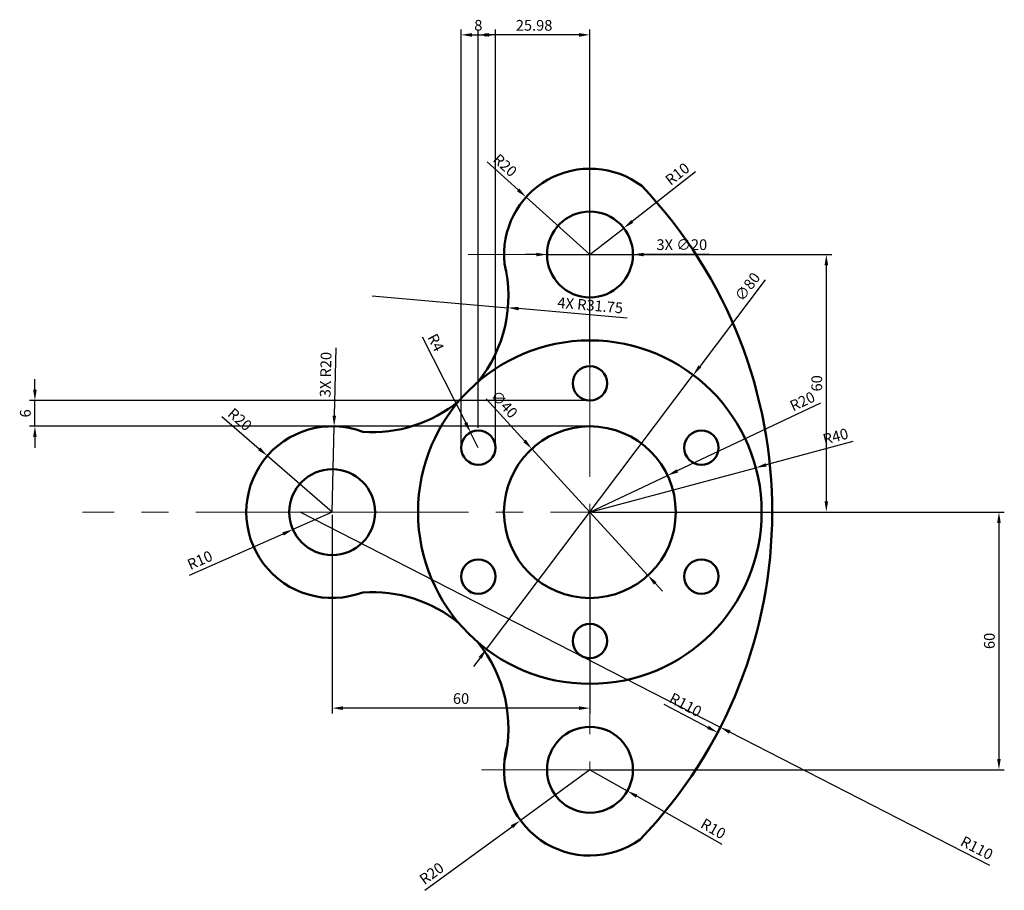
# Model space of a CAD drawing. Units: millimetres. Extents: x 4193 to 4422, y 3154 to 3357.
import ezdxf

# ---------------------------------------------------------------- set-up
doc = ezdxf.new("R2010")
doc.units = ezdxf.units.MM
doc.linetypes.add('CENTER', pattern=[50.8, 31.75, -6.35, 6.35, -6.35])
for name, color, linetype, lineweight in [('M-CNTR', 4, 'CENTER', 18), ('M-DIMS', 2, 'Continuous', 25), ('M-OUTL', 7, 'Continuous', 50)]:
    doc.layers.add(name, color=color, linetype=linetype, lineweight=lineweight)
doc.styles.get("Standard").update_dxf_attribs({"font": 'arial.ttf'})
doc.dimstyles.new('ISO-25', dxfattribs={"dimtxt": 2.5, "dimasz": 2.5, "dimexe": 1.25, "dimexo": 0.625, "dimtad": 1, "dimtxsty": 'Standard', "dimcen": 2.5, "dimadec": 0, "dimazin": 0, "dimtfac": 1, "dimtmove": 0, "dimatfit": 3, "dimfxl": 1, "dimarcsym": 0})

# ---------------------------------------------------------------- blocks, each defined once
blk = doc.blocks.new('*U1')
blk.add_circle((0, 0), 4)
blk = doc.blocks.new('*U2')
at = {"layer": 'M-OUTL', "color": 0, "linetype": 'ByBlock', "lineweight": -2, "transparency": 16777216}
for p, rotation in [((4325.57, 3272.51), 180), ((4299.59, 3257.51), 240), ((4351.55, 3257.51), 119.9999999999999), ((4299.59, 3227.51), 300), ((4351.55, 3227.51), 59.99999999999997)]:
    blk.add_blockref('*U1', p, dxfattribs=dict(at, rotation=rotation))
blk.add_blockref('*U1', (4325.57, 3212.51), dxfattribs=at)
blk = doc.blocks.new('*D3')
at = {"layer": 'Defpoints', "color": 0, "transparency": 16777216}
for p in [(4325.57, 3242.51), (4325.59, 3182.51), (4420.83, 3182.51)]:
    blk.add_point(p, dxfattribs=at)
at = {"layer": 'M-DIMS', "color": 0, "lineweight": -2, "transparency": 16777216}
for p, q in [((4326.2, 3242.51), (4422.08, 3242.51)), ((4420.83, 3240.01), (4420.83, 3185.01)), ((4326.22, 3182.51), (4422.08, 3182.51))]:
    blk.add_line(p, q, dxfattribs=at)
at = {"layer": 'M-DIMS', "color": 0, "transparency": 16777216}
for points in [[(4420.41, 3240.01), (4421.24, 3240.01), (4420.83, 3242.51)], [(4420.41, 3185.01), (4421.24, 3185.01), (4420.83, 3182.51)]]:
    blk.add_solid(points, dxfattribs=at)
at = {"layer": 'M-DIMS', "color": 0, "transparency": 16777216, "insert": (4418.92, 3212.51), "char_height": 2.5, "attachment_point": 5, "rotation": 90}
blk.add_mtext('60', dxfattribs=at)
blk = doc.blocks.new('*D4')
at = {"layer": 'Defpoints', "color": 0, "transparency": 16777216}
for p in [(4265.57, 3242.51), (4325.57, 3242.51), (4265.57, 3196.86)]:
    blk.add_point(p, dxfattribs=at)
at = {"layer": 'M-DIMS', "color": 0, "lineweight": -2, "transparency": 16777216}
for p, q in [((4265.57, 3241.88), (4265.57, 3195.61)), ((4325.57, 3241.88), (4325.57, 3195.61)), ((4323.07, 3196.86), (4268.07, 3196.86))]:
    blk.add_line(p, q, dxfattribs=at)
at = {"layer": 'M-DIMS', "color": 0, "transparency": 16777216}
for points in [[(4268.07, 3197.27), (4268.07, 3196.44), (4265.57, 3196.86)], [(4323.07, 3197.27), (4323.07, 3196.44), (4325.57, 3196.86)]]:
    blk.add_solid(points, dxfattribs=at)
at = {"layer": 'M-DIMS', "color": 0, "transparency": 16777216, "insert": (4295.57, 3198.76), "char_height": 2.5, "attachment_point": 5}
blk.add_mtext('60', dxfattribs=at)
blk = doc.blocks.new('*D5')
at = {"layer": 'Defpoints', "color": 0, "transparency": 16777216}
for p in [(4333.46, 3308.67), (4325.59, 3302.51)]:
    blk.add_point(p, dxfattribs=at)
at = {"layer": 'M-DIMS', "color": 0, "lineweight": -2, "transparency": 16777216}
for p, q in [((4350.15, 3321.75), (4335.43, 3310.22)), ((4325.59, 3302.51), (4333.46, 3308.67))]:
    blk.add_line(p, q, dxfattribs=at)
at = {"layer": 'M-DIMS', "color": 0, "transparency": 16777216}
blk.add_solid([(4335.18, 3310.54), (4335.69, 3309.89), (4333.46, 3308.67)], dxfattribs=at)
at = {"layer": 'M-DIMS', "color": 0, "transparency": 16777216, "insert": (4346.14, 3321.02), "char_height": 2.5, "attachment_point": 5, "rotation": 38.0842}
blk.add_mtext('R10', dxfattribs=at)
blk = doc.blocks.new('*D6')
at = {"layer": 'Defpoints', "color": 0, "transparency": 16777216}
for p in [(4310.73, 3315.89), (4325.59, 3302.51)]:
    blk.add_point(p, dxfattribs=at)
at = {"layer": 'M-DIMS', "color": 0, "lineweight": -2, "transparency": 16777216}
for p, q in [((4301.65, 3324.06), (4308.87, 3317.56)), ((4325.59, 3302.51), (4310.73, 3315.89))]:
    blk.add_line(p, q, dxfattribs=at)
at = {"layer": 'M-DIMS', "color": 0, "transparency": 16777216}
blk.add_solid([(4309.15, 3317.87), (4308.59, 3317.25), (4310.73, 3315.89)], dxfattribs=at)
at = {"layer": 'M-DIMS', "color": 0, "transparency": 16777216, "insert": (4305.6, 3323.06), "char_height": 2.5, "attachment_point": 5, "rotation": 318.016}
blk.add_mtext('R20', dxfattribs=at)
blk = doc.blocks.new('*D7')
at = {"layer": 'Defpoints', "color": 0, "transparency": 16777216}
for p in [(4364.21, 3252.86), (4325.57, 3242.51)]:
    blk.add_point(p, dxfattribs=at)
at = {"layer": 'M-DIMS', "color": 0, "lineweight": -2, "transparency": 16777216}
for p, q in [((4386.84, 3258.93), (4366.62, 3253.51)), ((4325.57, 3242.51), (4364.21, 3252.86))]:
    blk.add_line(p, q, dxfattribs=at)
at = {"layer": 'M-DIMS', "color": 0, "transparency": 16777216}
blk.add_solid([(4366.51, 3253.91), (4366.73, 3253.11), (4364.21, 3252.86)], dxfattribs=at)
at = {"layer": 'M-DIMS', "color": 0, "transparency": 16777216, "insert": (4382.86, 3259.83), "char_height": 2.5, "attachment_point": 5, "rotation": 15.0027}
blk.add_mtext('R40', dxfattribs=at)
blk = doc.blocks.new('*D8')
at = {"layer": 'Defpoints', "color": 0, "transparency": 16777216}
for p in [(4343.66, 3251.04), (4325.57, 3242.51)]:
    blk.add_point(p, dxfattribs=at)
at = {"layer": 'M-DIMS', "color": 0, "lineweight": -2, "transparency": 16777216}
for p, q in [((4379.26, 3267.85), (4345.92, 3252.11)), ((4325.57, 3242.51), (4343.66, 3251.04))]:
    blk.add_line(p, q, dxfattribs=at)
at = {"layer": 'M-DIMS', "color": 0, "transparency": 16777216}
blk.add_solid([(4345.74, 3252.49), (4346.1, 3251.73), (4343.66, 3251.04)], dxfattribs=at)
at = {"layer": 'M-DIMS', "color": 0, "transparency": 16777216, "insert": (4375.19, 3268.03), "char_height": 2.5, "attachment_point": 5, "rotation": 25.2677}
blk.add_mtext('R20', dxfattribs=at)
blk = doc.blocks.new('*D9')
at = {"layer": 'Defpoints', "color": 0, "transparency": 16777216}
for p in [(4297.79, 3261.08), (4299.59, 3257.51)]:
    blk.add_point(p, dxfattribs=at)
at = {"layer": 'M-DIMS', "color": 0, "lineweight": -2, "transparency": 16777216}
for p, q in [((4286.54, 3283.36), (4296.66, 3263.31)), ((4299.59, 3257.51), (4297.79, 3261.08))]:
    blk.add_line(p, q, dxfattribs=at)
at = {"layer": 'M-DIMS', "color": 0, "transparency": 16777216}
blk.add_solid([(4297.03, 3263.5), (4296.29, 3263.12), (4297.79, 3261.08)], dxfattribs=at)
at = {"layer": 'M-DIMS', "color": 0, "transparency": 16777216, "insert": (4289.4, 3281.85), "char_height": 2.5, "attachment_point": 5, "rotation": 296.7817}
blk.add_mtext('R4', dxfattribs=at)
blk = doc.blocks.new('*D10')
at = {"layer": 'Defpoints', "color": 0, "transparency": 16777216}
for p in [(4265.57, 3242.51), (4256.42, 3238.46)]:
    blk.add_point(p, dxfattribs=at)
at = {"layer": 'M-DIMS', "color": 0, "lineweight": -2, "transparency": 16777216}
for p, q in [((4265.57, 3242.51), (4256.42, 3238.46)), ((4232.36, 3227.82), (4254.14, 3237.45))]:
    blk.add_line(p, q, dxfattribs=at)
at = {"layer": 'M-DIMS', "color": 0, "transparency": 16777216}
blk.add_solid([(4253.97, 3237.83), (4254.31, 3237.07), (4256.42, 3238.46)], dxfattribs=at)
at = {"layer": 'M-DIMS', "color": 0, "transparency": 16777216, "insert": (4234.89, 3231.02), "char_height": 2.5, "attachment_point": 5, "rotation": 23.8595}
blk.add_mtext('R10', dxfattribs=at)
blk = doc.blocks.new('*D11')
at = {"layer": 'Defpoints', "color": 0, "transparency": 16777216}
for p in [(4250.46, 3255.61), (4265.57, 3242.51)]:
    blk.add_point(p, dxfattribs=at)
at = {"layer": 'M-DIMS', "color": 0, "lineweight": -2, "transparency": 16777216}
for p, q in [((4239.88, 3264.78), (4248.57, 3257.25)), ((4265.57, 3242.51), (4250.46, 3255.61))]:
    blk.add_line(p, q, dxfattribs=at)
at = {"layer": 'M-DIMS', "color": 0, "transparency": 16777216}
blk.add_solid([(4248.84, 3257.56), (4248.3, 3256.93), (4250.46, 3255.61)], dxfattribs=at)
at = {"layer": 'M-DIMS', "color": 0, "transparency": 16777216, "insert": (4243.86, 3263.85), "char_height": 2.5, "attachment_point": 5, "rotation": 319.0732}
blk.add_mtext('R20', dxfattribs=at)
blk = doc.blocks.new('*D12')
at = {"layer": 'Defpoints', "color": 0, "transparency": 16777216}
for p in [(4258.02, 3242.57), (4355.29, 3191.2)]:
    blk.add_point(p, dxfattribs=at)
at = {"layer": 'M-DIMS', "color": 0, "lineweight": -2, "transparency": 16777216}
blk.add_line((4342.77, 3197.81), (4353.08, 3192.37), dxfattribs=at)
at = {"layer": 'M-DIMS', "color": 0, "transparency": 16777216}
blk.add_solid([(4353.27, 3192.74), (4352.88, 3192), (4355.29, 3191.2)], dxfattribs=at)
at = {"layer": 'M-DIMS', "color": 0, "transparency": 16777216, "insert": (4347.7, 3197.35), "char_height": 2.5, "attachment_point": 5, "rotation": 332.1578}
blk.add_mtext('R110', dxfattribs=at)
blk = doc.blocks.new('*D13')
at = {"layer": 'Defpoints', "color": 0, "transparency": 16777216}
for p in [(4325.59, 3182.51), (4334.29, 3177.57)]:
    blk.add_point(p, dxfattribs=at)
at = {"layer": 'M-DIMS', "color": 0, "lineweight": -2, "transparency": 16777216}
for p, q in [((4325.59, 3182.51), (4334.29, 3177.57)), ((4356.35, 3165.06), (4336.47, 3176.34))]:
    blk.add_line(p, q, dxfattribs=at)
at = {"layer": 'M-DIMS', "color": 0, "transparency": 16777216}
blk.add_solid([(4336.67, 3176.7), (4336.26, 3175.98), (4334.29, 3177.57)], dxfattribs=at)
at = {"layer": 'M-DIMS', "color": 0, "transparency": 16777216, "insert": (4354.15, 3168.5), "char_height": 2.5, "attachment_point": 5, "rotation": 330.4382}
blk.add_mtext('R10', dxfattribs=at)
blk = doc.blocks.new('*D14')
at = {"layer": 'Defpoints', "color": 0, "transparency": 16777216}
for p in [(4325.57, 3182.51), (4309.42, 3170.71)]:
    blk.add_point(p, dxfattribs=at)
at = {"layer": 'M-DIMS', "color": 0, "lineweight": -2, "transparency": 16777216}
for p, q in [((4325.57, 3182.51), (4309.42, 3170.71)), ((4287.1, 3154.42), (4307.4, 3169.24))]:
    blk.add_line(p, q, dxfattribs=at)
at = {"layer": 'M-DIMS', "color": 0, "transparency": 16777216}
blk.add_solid([(4307.15, 3169.58), (4307.64, 3168.9), (4309.42, 3170.71)], dxfattribs=at)
at = {"layer": 'M-DIMS', "color": 0, "transparency": 16777216, "insert": (4288.9, 3158.09), "char_height": 2.5, "attachment_point": 5, "rotation": 36.1328}
blk.add_mtext('R20', dxfattribs=at)
blk = doc.blocks.new('MOUNTING-HOLE-D20')
blk.add_circle((10, 10), 10)
blk = doc.blocks.new('*D16')
at = {"layer": 'Defpoints', "color": 0, "transparency": 16777216}
for p in [(4325.59, 3302.51), (4325.57, 3242.51), (4380.63, 3242.51)]:
    blk.add_point(p, dxfattribs=at)
at = {"layer": 'M-DIMS', "color": 0, "lineweight": -2, "transparency": 16777216}
for p, q in [((4326.22, 3302.51), (4381.88, 3302.51)), ((4380.63, 3300.01), (4380.63, 3245.01)), ((4326.2, 3242.51), (4381.88, 3242.51))]:
    blk.add_line(p, q, dxfattribs=at)
at = {"layer": 'M-DIMS', "color": 0, "transparency": 16777216}
for points in [[(4380.22, 3300.01), (4381.05, 3300.01), (4380.63, 3302.51)], [(4380.22, 3245.01), (4381.05, 3245.01), (4380.63, 3242.51)]]:
    blk.add_solid(points, dxfattribs=at)
at = {"layer": 'M-DIMS', "color": 0, "transparency": 16777216, "insert": (4378.73, 3272.51), "char_height": 2.5, "attachment_point": 5, "rotation": 90}
blk.add_mtext('60', dxfattribs=at)
blk = doc.blocks.new('*D17')
at = {"layer": 'Defpoints', "color": 0, "transparency": 16777216}
for p in [(4196.34, 3268.51), (4325.57, 3268.51), (4325.57, 3262.51)]:
    blk.add_point(p, dxfattribs=at)
at = {"layer": 'M-DIMS', "color": 0, "lineweight": -2, "transparency": 16777216}
for p, q in [((4196.34, 3271.01), (4196.34, 3273.51)), ((4324.95, 3268.51), (4195.09, 3268.51)), ((4196.34, 3262.51), (4196.34, 3268.51)), ((4324.95, 3262.51), (4195.09, 3262.51)), ((4196.34, 3260.01), (4196.34, 3257.51))]:
    blk.add_line(p, q, dxfattribs=at)
at = {"layer": 'M-DIMS', "color": 0, "transparency": 16777216}
for points in [[(4195.92, 3271.01), (4196.75, 3271.01), (4196.34, 3268.51)], [(4195.92, 3260.01), (4196.75, 3260.01), (4196.34, 3262.51)]]:
    blk.add_solid(points, dxfattribs=at)
at = {"layer": 'M-DIMS', "color": 0, "transparency": 16777216, "insert": (4194.43, 3265.51), "char_height": 2.5, "attachment_point": 5, "rotation": 90}
blk.add_mtext('6', dxfattribs=at)
blk = doc.blocks.new('*D18')
at = {"layer": 'Defpoints', "color": 0, "transparency": 16777216}
for p in [(4299.59, 3353.67), (4325.57, 3276.51), (4299.59, 3261.51)]:
    blk.add_point(p, dxfattribs=at)
at = {"layer": 'M-DIMS', "color": 0, "lineweight": -2, "transparency": 16777216}
for p, q in [((4299.59, 3262.13), (4299.59, 3354.92)), ((4325.57, 3277.13), (4325.57, 3354.92)), ((4323.07, 3353.67), (4302.09, 3353.67))]:
    blk.add_line(p, q, dxfattribs=at)
at = {"layer": 'M-DIMS', "color": 0, "transparency": 16777216}
for points in [[(4302.09, 3354.08), (4302.09, 3353.25), (4299.59, 3353.67)], [(4323.07, 3354.08), (4323.07, 3353.25), (4325.57, 3353.67)]]:
    blk.add_solid(points, dxfattribs=at)
at = {"layer": 'M-DIMS', "color": 0, "transparency": 16777216, "insert": (4312.58, 3355.57), "char_height": 2.5, "attachment_point": 5}
blk.add_mtext('25.98', dxfattribs=at)
blk = doc.blocks.new('*D19')
at = {"layer": 'Defpoints', "color": 0, "transparency": 16777216}
for p in [(4303.59, 3353.67), (4295.59, 3257.51), (4303.59, 3257.51)]:
    blk.add_point(p, dxfattribs=at)
at = {"layer": 'M-DIMS', "color": 0, "lineweight": -2, "transparency": 16777216}
for p, q in [((4295.59, 3258.13), (4295.59, 3354.92)), ((4303.59, 3258.13), (4303.59, 3354.92)), ((4298.09, 3353.67), (4301.09, 3353.67))]:
    blk.add_line(p, q, dxfattribs=at)
at = {"layer": 'M-DIMS', "color": 0, "transparency": 16777216}
for points in [[(4298.09, 3354.08), (4298.09, 3353.25), (4295.59, 3353.67)], [(4301.09, 3354.08), (4301.09, 3353.25), (4303.59, 3353.67)]]:
    blk.add_solid(points, dxfattribs=at)
at = {"layer": 'M-DIMS', "color": 0, "transparency": 16777216, "insert": (4299.59, 3355.57), "char_height": 2.5, "attachment_point": 5}
blk.add_mtext('8', dxfattribs=at)
blk = doc.blocks.new('*D20')
at = {"layer": 'Defpoints', "color": 0, "transparency": 16777216}
for p in [(4266, 3262.5), (4265.57, 3242.51)]:
    blk.add_point(p, dxfattribs=at)
at = {"layer": 'M-DIMS', "color": 0, "lineweight": -2, "transparency": 16777216}
for p, q in [((4266.39, 3280.79), (4266.05, 3265)), ((4265.57, 3242.51), (4266, 3262.5))]:
    blk.add_line(p, q, dxfattribs=at)
at = {"layer": 'M-DIMS', "color": 0, "transparency": 16777216}
blk.add_solid([(4265.64, 3265.01), (4266.47, 3264.99), (4266, 3262.5)], dxfattribs=at)
at = {"layer": 'M-DIMS', "color": 0, "transparency": 16777216, "insert": (4264.36, 3274.54), "char_height": 2.5, "attachment_point": 5, "rotation": 88.7678}
blk.add_mtext('3X R20', dxfattribs=at)
blk = doc.blocks.new('*D21')
at = {"layer": 'Defpoints', "color": 0, "transparency": 16777216}
for p in [(4274.85, 3292.87), (4306.48, 3290.12)]:
    blk.add_point(p, dxfattribs=at)
at = {"layer": 'M-DIMS', "color": 0, "lineweight": -2, "transparency": 16777216}
for p, q in [((4274.85, 3292.87), (4306.48, 3290.12)), ((4334.22, 3287.71), (4308.97, 3289.91))]:
    blk.add_line(p, q, dxfattribs=at)
at = {"layer": 'M-DIMS', "color": 0, "transparency": 16777216}
blk.add_solid([(4309.01, 3290.32), (4308.94, 3289.49), (4306.48, 3290.12)], dxfattribs=at)
at = {"layer": 'M-DIMS', "color": 0, "transparency": 16777216, "insert": (4325.63, 3290.37), "char_height": 2.5, "attachment_point": 5, "rotation": 355.0338}
blk.add_mtext('4X R31.75', dxfattribs=at)
blk = doc.blocks.new('*D22')
at = {"layer": 'Defpoints', "color": 0, "transparency": 16777216}
for p in [(4258.02, 3242.57), (4355.92, 3192.42)]:
    blk.add_point(p, dxfattribs=at)
at = {"layer": 'M-DIMS', "color": 0, "lineweight": -2, "transparency": 16777216}
for p, q in [((4258.02, 3242.57), (4355.92, 3192.42)), ((4418.73, 3160.23), (4358.14, 3191.28))]:
    blk.add_line(p, q, dxfattribs=at)
at = {"layer": 'M-DIMS', "color": 0, "transparency": 16777216}
blk.add_solid([(4358.33, 3191.65), (4357.95, 3190.91), (4355.92, 3192.42)], dxfattribs=at)
at = {"layer": 'M-DIMS', "color": 0, "transparency": 16777216, "insert": (4415.53, 3164.01), "char_height": 2.5, "attachment_point": 5, "rotation": 332.8725}
blk.add_mtext('R110', dxfattribs=at)
blk = doc.blocks.new('*D23')
at = {"layer": 'Defpoints', "color": 0, "transparency": 16777216}
for p in [(4315.59, 3302.51), (4335.59, 3302.51)]:
    blk.add_point(p, dxfattribs=at)
at = {"layer": 'M-DIMS', "color": 0, "lineweight": -2, "transparency": 16777216}
for p, q in [((4313.09, 3302.51), (4310.59, 3302.51)), ((4315.59, 3302.51), (4335.59, 3302.51)), ((4353.37, 3302.51), (4338.09, 3302.51))]:
    blk.add_line(p, q, dxfattribs=at)
at = {"layer": 'M-DIMS', "color": 0, "transparency": 16777216}
for points in [[(4313.09, 3302.92), (4313.09, 3302.09), (4315.59, 3302.51)], [(4338.09, 3302.92), (4338.09, 3302.09), (4335.59, 3302.51)]]:
    blk.add_solid(points, dxfattribs=at)
at = {"layer": 'M-DIMS', "color": 0, "transparency": 16777216, "insert": (4346.98, 3304.48), "char_height": 2.5, "attachment_point": 5, "rotation": 0.0026}
blk.add_mtext('3X ∅20', dxfattribs=at)
blk = doc.blocks.new('*D24')
at = {"layer": 'Defpoints', "color": 0, "transparency": 16777216}
for p in [(4312.05, 3257.24), (4339.09, 3227.77)]:
    blk.add_point(p, dxfattribs=at)
at = {"layer": 'M-DIMS', "color": 0, "lineweight": -2, "transparency": 16777216}
for p, q in [((4301.39, 3268.87), (4310.36, 3259.09)), ((4339.09, 3227.77), (4312.05, 3257.24)), ((4340.78, 3225.93), (4342.47, 3224.08))]:
    blk.add_line(p, q, dxfattribs=at)
at = {"layer": 'M-DIMS', "color": 0, "transparency": 16777216}
for points in [[(4310.67, 3259.37), (4310.05, 3258.81), (4312.05, 3257.24)], [(4341.09, 3226.21), (4340.47, 3225.64), (4339.09, 3227.77)]]:
    blk.add_solid(points, dxfattribs=at)
at = {"layer": 'M-DIMS', "color": 0, "transparency": 16777216, "insert": (4305.39, 3267.42), "char_height": 2.5, "attachment_point": 5, "rotation": 312.5304}
blk.add_mtext('∅40', dxfattribs=at)
blk = doc.blocks.new('*D25')
at = {"layer": 'Defpoints', "color": 0, "transparency": 16777216}
for p in [(4349.65, 3274.45), (4301.49, 3210.57)]:
    blk.add_point(p, dxfattribs=at)
at = {"layer": 'M-DIMS', "color": 0, "lineweight": -2, "transparency": 16777216}
for p, q in [((4366.37, 3296.62), (4351.15, 3276.44)), ((4301.49, 3210.57), (4349.65, 3274.45)), ((4299.99, 3208.57), (4298.48, 3206.57))]:
    blk.add_line(p, q, dxfattribs=at)
at = {"layer": 'M-DIMS', "color": 0, "transparency": 16777216}
for points in [[(4350.82, 3276.69), (4351.49, 3276.19), (4349.65, 3274.45)], [(4299.65, 3208.82), (4300.32, 3208.32), (4301.49, 3210.57)]]:
    blk.add_solid(points, dxfattribs=at)
at = {"layer": 'M-DIMS', "color": 0, "transparency": 16777216, "insert": (4362.52, 3294.8), "char_height": 2.5, "attachment_point": 5, "rotation": 52.99}
blk.add_mtext('∅80', dxfattribs=at)

msp = doc.modelspace()

# ---------------------------------------------------------------- linework, layer by layer
at = {"layer": 'M-CNTR'}
for p, q in [((4325.57, 3282.507), (4325.57, 3342.565)), ((4297.227, 3302.507), (4369.532, 3302.507)), ((4325.57, 3282.507), (4325.57, 3202.507)), ((4265.57, 3242.507), (4207.436, 3242.507)), ((4265.57, 3242.507), (4365.57, 3242.507)), ((4325.57, 3222.507), (4325.57, 3182.507)), ((4300.344, 3182.507), (4360.048, 3182.507))]:
    msp.add_line(p, q, dxfattribs=at)
at = {"layer": 'M-OUTL'}
for radius in [40, 20]:
    msp.add_circle((4325.57, 3242.507), radius, dxfattribs=at)
for centre, radius, start, end in [((4325.594, 3302.507), 20, 52.95426, 186.19719), ((4258.02, 3242.574), 110, 316.08576, 43.62719), ((4274.851, 3292.872), 31.752, 320.82747, 13.61765), ((4274.851, 3292.872), 31.752, 266.11346, 309.5733), ((4265.57, 3242.507), 20, 69.11755, 290.88245), ((4274.851, 3192.141), 31.752, 50.4267, 93.88654), ((4274.851, 3192.141), 31.752, 346.38235, 39.17253), ((4325.57, 3182.507), 20, 164.19958, 305.77319), ((4325.57, 3182.507), 20, 164.19958, 305.77319)]:
    msp.add_arc(centre, radius, start, end, dxfattribs=at)

# ---------------------------------------------------------------- block references
for name, p in [('MOUNTING-HOLE-D20', (4315.594, 3292.507)), ('*U2', (0, 0)), ('MOUNTING-HOLE-D20', (4255.57, 3232.507)), ('MOUNTING-HOLE-D20', (4315.594, 3172.507))]:
    msp.add_blockref(name, p, dxfattribs=at)

# ---------------------------------------------------------------- dimensions: what is measured, and where the dimension line sits
at = {"layer": 'M-DIMS'}
for base, p1, p2, override, picture, middle in [((4303.589, 3353.665), (4295.589, 3257.507), (4303.589, 3257.507), {"dimdec": 0, "dimlfac": 1, "dimrnd": 0, "dimzin": 0, "dimdsep": 46, "dimlunit": 2}, '*D19', (4299.589, 3355.567)), ((4299.589, 3353.665), (4325.57, 3276.507), (4299.589, 3261.507), {"dimdec": 2, "dimlfac": 1, "dimrnd": 0, "dimzin": 0, "dimdsep": 46, "dimlunit": 2}, '*D18', (4312.58, 3355.567)), ((4265.57, 3196.857), (4325.57, 3242.507), (4265.57, 3242.507), {"dimclrd": 0, "dimclre": 0, "dimclrt": 0}, '*D4', (4295.57, 3198.759))]:
    dim = msp.add_linear_dim(base=base, p1=p1, p2=p2, dimstyle='ISO-25', override=override, dxfattribs=at)
    dim.commit()
    dim.dimension.update_dxf_attribs({"geometry": picture, "text_midpoint": middle})
dim = msp.add_radius_dim(center=(4325.594, 3302.507), mpoint=(4310.727, 3315.885), dimstyle='ISO-25', override={"dimclrd": 0, "dimclre": 0, "dimclrt": 0}, dxfattribs=at)
dim.commit()
dim.dimension.update_dxf_attribs({"geometry": '*D6', "text_midpoint": (4305.601, 3323.056)})
for center, mpoint, override, picture, middle in [((4325.594, 3302.507), (4333.465, 3308.675), {"dimclrd": 0, "dimclre": 0, "dimclrt": 0}, '*D5', (4347.313, 3319.527)), ((4299.589, 3257.507), (4297.787, 3261.077), {"dimclrd": 0, "dimclre": 0, "dimclrt": 0}, '*D9', (4287.727, 3281.009)), ((4325.57, 3242.507), (4343.657, 3251.044), {"dimclrd": 0, "dimclre": 0, "dimclrt": 0}, '*D8', (4376, 3266.31)), ((4265.57, 3242.507), (4250.459, 3255.608), {"dimclrd": 0, "dimclre": 0, "dimclrt": 0}, '*D11', (4242.61, 3262.414)), ((4325.57, 3242.507), (4364.207, 3252.861), {"dimclrd": 0, "dimclre": 0, "dimclrt": 0}, '*D7', (4383.356, 3257.993)), ((4265.57, 3242.507), (4256.425, 3238.462), {"dimclrd": 0, "dimclre": 0, "dimclrt": 0}, '*D10', (4235.66, 3229.278)), ((4258.02, 3242.574), (4355.286, 3191.2), {"dimclrd": 0, "dimclre": 0, "dimclrt": 0}, '*D12', (4346.816, 3195.673)), ((4258.02, 3242.574), (4355.919, 3192.417), {"dimdec": 0, "dimlfac": 1, "dimrnd": 0, "dimzin": 0, "dimdsep": 46, "dimlunit": 2}, '*D22', (4414.659, 3162.322)), ((4325.57, 3182.507), (4309.417, 3170.713), {"dimclrd": 0, "dimclre": 0, "dimclrt": 0}, '*D14', (4290.017, 3156.55)), ((4325.594, 3182.507), (4334.292, 3177.573), {"dimclrd": 0, "dimclre": 0, "dimclrt": 0}, '*D13', (4353.212, 3166.842))]:
    dim = msp.add_radius_dim(center=center, mpoint=mpoint, dimstyle='ISO-25', override=override, dxfattribs=at)
    dim.commit()
    dim.dimension.update_dxf_attribs({"geometry": picture, "text_midpoint": middle, "dimtype": 164})
dim = msp.add_diameter_dim_2p(p1=(4315.594, 3302.506), p2=(4335.594, 3302.507), text='3X <>', dimstyle='ISO-25', override={"dimdec": 0, "dimlfac": 1, "dimrnd": 0, "dimzin": 0, "dimdsep": 46, "dimlunit": 2}, dxfattribs=at)
dim.commit()
dim.dimension.update_dxf_attribs({"geometry": '*D23', "text_midpoint": (4346.984, 3302.508)})
for base, p1, p2, override, picture, middle in [((4380.632, 3242.507), (4325.594, 3302.507), (4325.57, 3242.507), {"dimdec": 0, "dimlfac": 1, "dimrnd": 0, "dimzin": 0, "dimdsep": 46, "dimlunit": 2}, '*D16', (4378.731, 3272.507)), ((4196.336, 3268.507), (4325.57, 3262.507), (4325.57, 3268.507), {"dimdec": 0, "dimlfac": 1, "dimrnd": 0, "dimzin": 0, "dimdsep": 46, "dimlunit": 2}, '*D17', (4194.435, 3265.507)), ((4420.825, 3182.507), (4325.57, 3242.507), (4325.594, 3182.507), {"dimclrd": 0, "dimclre": 0, "dimclrt": 0}, '*D3', (4418.924, 3212.507))]:
    dim = msp.add_linear_dim(base=base, p1=p1, p2=p2, angle=90, dimstyle='ISO-25', override=override, dxfattribs=at)
    dim.commit()
    dim.dimension.update_dxf_attribs({"geometry": picture, "text_midpoint": middle})
for p1, p2, picture, middle in [((4301.492, 3210.565), (4349.648, 3274.448), '*D25', (4364.095, 3293.613)), ((4339.09, 3227.768), (4312.051, 3257.245), '*D24', (4303.939, 3266.088))]:
    dim = msp.add_diameter_dim_2p(p1=p1, p2=p2, dimstyle='ISO-25', override={"dimdec": 0, "dimlfac": 1, "dimrnd": 0, "dimzin": 0, "dimdsep": 46, "dimlunit": 2}, dxfattribs=at)
    dim.commit()
    dim.dimension.update_dxf_attribs({"geometry": picture, "text_midpoint": middle, "dimtype": 163})
for center, mpoint, text, override, picture, middle in [((4274.851, 3292.872), (4306.484, 3290.123), '4X <>', {"dimdec": 2, "dimlfac": 1, "dimrnd": 0, "dimzin": 0, "dimdsep": 46, "dimlunit": 2}, '*D21', (4325.464, 3288.474)), ((4265.57, 3242.507), (4266, 3262.502), '3X <>', {"dimdec": 0, "dimlfac": 1, "dimrnd": 0, "dimzin": 0, "dimdsep": 46, "dimlunit": 2}, '*D20', (4266.258, 3274.499))]:
    dim = msp.add_radius_dim(center=center, mpoint=mpoint, text=text, dimstyle='ISO-25', override=override, dxfattribs=at)
    dim.commit()
    dim.dimension.update_dxf_attribs({"geometry": picture, "text_midpoint": middle, "dimtype": 164})

doc.saveas('drawing.dxf')
